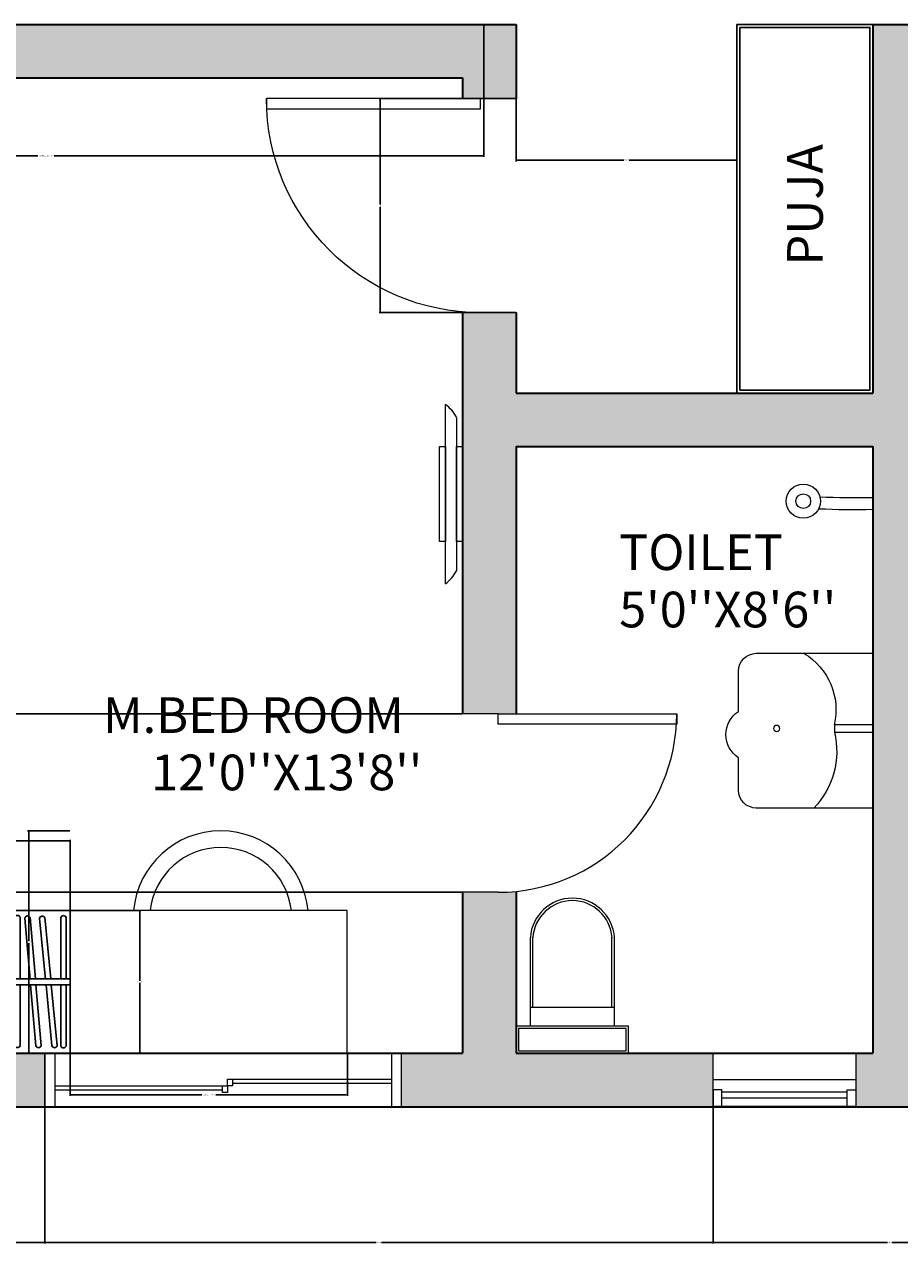
# Model space of a CAD drawing. Units: inches. Extents: x 1789 to 2841, y 3180 to 3702.
# Tile 9 of 14: x 2477 to 2624, y 3180 to 3385. Entities that reach past the tile are written whole.
import ezdxf

# ---------------------------------------------------------------- set-up
doc = ezdxf.new("R2010")
doc.units = ezdxf.units.IN
doc.header["$MEASUREMENT"] = 0
for name, color, linetype, lineweight in [('A-ANNO-DIMS', 2, 'Continuous', 18), ('A-AREA-IDEN', 7, 'Continuous', 18), ('A-EQPM', 8, 'Continuous', 18), ('A-FLOR-CASE', 34, 'Continuous', 25), ('A-FLOR-FIXT', 9, 'Continuous', 18), ('A-WALL', 40, 'Continuous', 35), ('A-WALL-PATT', 252, 'Continuous', 13), ('DORS', 70, 'Continuous', 18), ('FURNITURE', 34, 'Continuous', 18), ('WINDOWS', 130, 'Continuous', 18)]:
    doc.layers.add(name, color=color, linetype=linetype, lineweight=lineweight)
doc.styles.get("Standard").update_dxf_attribs({"font": 'arial.ttf'})
doc.dimstyles.get("Standard").update_dxf_attribs({"dimtxt": 0.18, "dimasz": 0.18, "dimexe": 0.18, "dimexo": 0.0625, "dimgap": 0.09, "dimtad": 0, "dimtih": 1, "dimtoh": 1, "dimdec": 0, "dimzin": 0, "dimdsep": 46, "dimlunit": 3, "dimtxsty": 'Standard', "dimcen": 0.09, "dimadec": 0, "dimazin": 0, "dimtfac": 1, "dimtdec": 0, "dimtofl": 0, "dimtmove": 0, "dimatfit": 3, "dimfxl": 1, "dimtolj": 1, "dimtzin": 0, "dimarcsym": 0})

# ---------------------------------------------------------------- blocks, each defined once
blk = doc.blocks.new('CUBOARD')
for p, q in [((2183.73, 3646.16), (2183.73, 3568.16)), ((2184.71, 3646.16), (2184.71, 3568.16))]:
    blk.add_line(p, q)
blk.add_lwpolyline([(2172.23, 3646.16), (2196.23, 3646.16), (2196.23, 3568.16), (2172.23, 3568.16)], close=True)
for points in [[(2195.39, 3645.6), (2184.67, 3644.55)], [(2183.69, 3644.46), (2173.95, 3643.51)], [(2173.97, 3642.61), (2183.78, 3643.57)], [(2184.76, 3643.66), (2195.54, 3644.71)], [(2195.78, 3645.16), (2195.78, 3645.18)], [(2183.73, 3641.98), (2173.93, 3641.98)], [(2195.47, 3641.98), (2184.71, 3641.98)], [(2195.82, 3641.5), (2195.82, 3641.53)], [(2173.86, 3641.08), (2183.73, 3641.08)], [(2183.76, 3639.46), (2173.96, 3640.08)], [(2184.71, 3641.08), (2195.53, 3641.08)], [(2195.45, 3638.71), (2184.74, 3639.4)], [(2173.84, 3639.19), (2183.7, 3638.57)], [(2184.68, 3638.5), (2195.46, 3637.81)], [(2195.77, 3638.22), (2195.78, 3638.24)], [(2173.83, 3635.92), (2183.73, 3635.92)], [(2183.73, 3636.82), (2173.9, 3636.82)], [(2195.43, 3636.82), (2184.71, 3636.82)], [(2184.71, 3635.92), (2195.5, 3635.92)], [(2195.78, 3636.35), (2195.78, 3636.37)], [(2173.81, 3633.34), (2183.73, 3633.34)], [(2183.73, 3634.24), (2173.88, 3634.24)], [(2195.42, 3634.24), (2184.71, 3634.24)], [(2184.71, 3633.34), (2195.48, 3633.34)], [(2195.77, 3633.77), (2195.77, 3633.79)], [(2183.73, 3631.66), (2173.86, 3631.66)], [(2195.4, 3631.66), (2184.71, 3631.66)], [(2195.75, 3631.19), (2195.75, 3631.21)], [(2173.8, 3630.76), (2183.73, 3630.76)], [(2184.71, 3630.76), (2195.47, 3630.76)], [(2173.78, 3628.19), (2183.73, 3628.19)], [(2183.73, 3629.08), (2173.85, 3629.08)], [(2183.8, 3626.57), (2173.93, 3627.31)], [(2195.38, 3629.08), (2184.71, 3629.08)], [(2184.71, 3628.19), (2195.45, 3628.19)], [(2195.73, 3628.61), (2195.73, 3628.63)], [(2173.79, 3626.43), (2183.74, 3625.68)], [(2184.71, 3625.61), (2195.4, 3624.81)], [(2195.4, 3625.7), (2184.78, 3626.5)], [(2195.72, 3625.21), (2195.72, 3625.23)], [(2173.75, 3623.03), (2183.73, 3623.03)], [(2183.73, 3623.92), (2173.81, 3623.92)], [(2195.35, 3623.92), (2184.71, 3623.92)], [(2184.71, 3623.03), (2195.42, 3623.03)], [(2195.7, 3623.45), (2195.7, 3623.48)], [(2183.73, 3621.34), (2173.8, 3621.34)], [(2195.33, 3621.34), (2184.71, 3621.34)], [(2173.73, 3620.45), (2183.73, 3620.45)], [(2195.22, 3619.57), (2184.65, 3618.76)], [(2184.71, 3620.45), (2195.4, 3620.45)], [(2195.6, 3619.13), (2195.6, 3619.15)], [(2195.68, 3620.87), (2195.68, 3620.9)], [(2183.67, 3618.69), (2173.75, 3617.93)], [(2173.75, 3617.03), (2183.74, 3617.8)], [(2184.71, 3617.87), (2195.35, 3618.68)], [(2173.7, 3615.29), (2183.73, 3615.29)], [(2183.73, 3616.19), (2173.77, 3616.19)], [(2195.3, 3616.19), (2184.71, 3616.19)], [(2184.71, 3615.29), (2195.37, 3615.29)], [(2195.65, 3615.71), (2195.65, 3615.74)], [(2173.68, 3612.71), (2183.73, 3612.71)], [(2183.73, 3613.61), (2173.75, 3613.61)], [(2195.28, 3613.61), (2184.71, 3613.61)], [(2184.71, 3612.71), (2195.35, 3612.71)], [(2195.63, 3613.14), (2195.63, 3613.16)], [(2173.67, 3611.18), (2183.69, 3610.23)], [(2183.78, 3611.12), (2173.82, 3612.07)], [(2195.26, 3610.03), (2184.75, 3611.03)], [(2184.67, 3610.14), (2195.24, 3609.13)], [(2195.23, 3608.76), (2184.7, 3608.45)], [(2195.56, 3609.53), (2195.57, 3609.55)], [(2173.66, 3607.23), (2183.75, 3607.53)], [(2183.72, 3608.42), (2173.71, 3608.13)], [(2184.73, 3607.55), (2195.33, 3607.87)], [(2195.6, 3608.3), (2195.6, 3608.32)], [(2173.63, 3604.98), (2183.73, 3604.98)], [(2183.73, 3605.87), (2173.7, 3605.87)], [(2195.23, 3605.87), (2184.71, 3605.87)], [(2184.71, 3604.98), (2195.3, 3604.98)], [(2195.58, 3605.4), (2195.58, 3605.42)], [(2183.73, 3603.29), (2173.68, 3603.29)], [(2195.22, 3603.29), (2184.71, 3603.29)], [(2195.57, 3602.82), (2195.57, 3602.84)], [(2173.61, 3602.4), (2183.73, 3602.4)], [(2183.73, 3600.71), (2173.67, 3600.71)], [(2184.71, 3602.4), (2195.28, 3602.4)], [(2195.2, 3600.71), (2184.71, 3600.71)], [(2173.6, 3599.82), (2183.73, 3599.82)], [(2184.71, 3599.82), (2195.27, 3599.82)], [(2195.55, 3600.24), (2195.55, 3600.27)], [(2173.58, 3597.24), (2183.73, 3597.24)], [(2183.73, 3598.13), (2173.65, 3598.13)], [(2195.18, 3598.13), (2184.71, 3598.13)], [(2184.71, 3597.24), (2195.25, 3597.24)], [(2195.53, 3597.66), (2195.53, 3597.69)], [(2173.56, 3595.36), (2183.71, 3594.72)], [(2183.77, 3595.62), (2173.68, 3596.25)], [(2184.69, 3594.66), (2195.19, 3594)], [(2195.18, 3594.9), (2184.74, 3595.55)], [(2195.5, 3594.4), (2195.5, 3594.43)], [(2183.73, 3592.98), (2173.62, 3592.98)], [(2195.15, 3592.98), (2184.71, 3592.98)], [(2195.5, 3592.5), (2195.5, 3592.53)], [(2173.55, 3592.08), (2183.73, 3592.08)], [(2173.57, 3590.49), (2183.74, 3589.59)], [(2183.73, 3590.49), (2173.72, 3591.37)], [(2184.71, 3592.08), (2195.22, 3592.08)], [(2195.17, 3589.47), (2184.71, 3590.4)], [(2184.71, 3589.5), (2195.16, 3588.58)], [(2195.48, 3588.97), (2195.48, 3589)], [(2173.51, 3586.92), (2183.73, 3586.92)], [(2183.73, 3587.82), (2173.58, 3587.82)], [(2194.84, 3586.83), (2184.58, 3585.23)], [(2195.12, 3587.82), (2184.71, 3587.82)], [(2184.71, 3586.92), (2195.19, 3586.92)], [(2195.26, 3586.41), (2195.25, 3586.44)], [(2195.47, 3587.35), (2195.47, 3587.37)], [(2183.61, 3585.08), (2173.56, 3583.51)], [(2173.63, 3582.62), (2183.75, 3584.19)], [(2184.71, 3584.34), (2195.04, 3585.95)], [(2183.73, 3582.66), (2173.55, 3582.66)], [(2195.08, 3582.66), (2184.71, 3582.66)], [(2195.43, 3582.19), (2195.43, 3582.21)], [(2173.48, 3581.77), (2183.73, 3581.77)], [(2183.73, 3580.08), (2173.53, 3580.08)], [(2184.71, 3581.77), (2195.15, 3581.77)], [(2195.07, 3580.08), (2184.71, 3580.08)], [(2173.46, 3579.19), (2183.73, 3579.19)], [(2184.71, 3579.19), (2195.14, 3579.19)], [(2195.42, 3579.61), (2195.42, 3579.63)], [(2173.45, 3576.61), (2183.73, 3576.61)], [(2183.73, 3577.5), (2173.52, 3577.5)], [(2194.92, 3575.81), (2184.64, 3574.92)], [(2195.05, 3577.5), (2184.71, 3577.5)], [(2184.71, 3576.61), (2195.12, 3576.61)], [(2195.4, 3577.03), (2195.4, 3577.05)], [(2183.66, 3574.84), (2173.46, 3573.95)], [(2173.47, 3573.05), (2183.74, 3573.94)], [(2184.71, 3574.03), (2195.06, 3574.93)], [(2195.31, 3575.37), (2195.31, 3575.4)], [(2183.65, 3572.24), (2173.45, 3571.25)], [(2194.88, 3573.34), (2184.63, 3572.34)], [(2184.71, 3571.45), (2195.04, 3572.46)], [(2195.28, 3572.91), (2195.27, 3572.93)], [(2173.47, 3570.35), (2183.74, 3571.35)], [(2183.73, 3569.77), (2173.47, 3569.77)], [(2195, 3569.77), (2184.71, 3569.77)], [(2173.4, 3568.87), (2183.73, 3568.87)], [(2184.71, 3568.87), (2195.07, 3568.87)], [(2195.35, 3569.29), (2195.35, 3569.32)]]:
    blk.add_lwpolyline(points)
for centre, start, end in [((2195.31, 3645.13), 7.0195, 80.386), ((2174.12, 3643.06), 110.7367, 251.6587), ((2195.31, 3645.13), 299.464, 4.1032), ((2174.06, 3641.52), 105.1753, 246.0974), ((2195.34, 3641.52), 1.4582, 74.8247), ((2195.34, 3641.52), 293.9026, 358.5418), ((2174.06, 3639.62), 101.5232, 242.4452), ((2195.3, 3638.26), 357.8061, 71.1726), ((2195.3, 3638.26), 290.2505, 354.8897), ((2174.02, 3636.36), 105.1753, 246.0974), ((2195.31, 3636.36), 1.4582, 74.8247), ((2195.31, 3636.36), 293.9026, 358.5418), ((2174.01, 3633.78), 105.1753, 246.0974), ((2195.29, 3633.78), 1.4582, 74.8247), ((2195.29, 3633.78), 293.9026, 358.5418), ((2173.99, 3631.2), 105.1753, 246.0974), ((2195.27, 3631.2), 1.4582, 74.8247), ((2195.27, 3631.2), 293.9026, 358.5418), ((2173.97, 3628.62), 105.1753, 246.0974), ((2174.02, 3626.85), 100.888, 241.81), ((2195.26, 3628.62), 1.4582, 74.8247), ((2195.26, 3628.62), 293.9026, 358.5418), ((2195.24, 3625.25), 357.1709, 70.5374), ((2195.24, 3625.25), 289.6153, 354.2545), ((2173.94, 3623.46), 105.1753, 246.0974), ((2195.22, 3623.46), 1.4582, 74.8247), ((2195.22, 3623.46), 293.9026, 358.5418), ((2173.92, 3620.88), 105.1753, 246.0974), ((2195.21, 3620.88), 1.4582, 74.8247), ((2195.13, 3619.1), 5.8369, 79.2034), ((2195.13, 3619.1), 298.2814, 2.9206), ((2195.21, 3620.88), 293.9026, 358.5418), ((2173.9, 3617.48), 109.5541, 250.4761), ((2173.89, 3615.73), 105.1753, 246.0974), ((2195.17, 3615.73), 1.4582, 74.8247), ((2195.17, 3615.73), 293.9026, 358.5418), ((2173.87, 3613.15), 105.1753, 246.0974), ((2195.16, 3613.15), 1.4582, 74.8247), ((2195.16, 3613.15), 293.9026, 358.5418), ((2173.9, 3611.6), 99.7479, 240.6699), ((2195.12, 3608.3), 3.1408, 76.5073), ((2195.09, 3609.58), 288.4752, 353.1144), ((2195.09, 3609.58), 356.0307, 69.3973), ((2173.84, 3607.67), 106.858, 247.78), ((2195.12, 3608.3), 295.5853, 0.2245), ((2173.82, 3605.41), 105.1753, 246.0974), ((2195.11, 3605.41), 1.4582, 74.8247), ((2195.11, 3605.41), 293.9026, 358.5418), ((2173.81, 3602.83), 105.1753, 246.0974), ((2195.09, 3602.83), 1.4582, 74.8247), ((2195.09, 3602.83), 293.9026, 358.5418), ((2173.79, 3600.25), 105.1753, 246.0974), ((2195.08, 3600.25), 1.4582, 74.8247), ((2195.08, 3600.25), 293.9026, 358.5418), ((2173.77, 3597.67), 105.1753, 246.0974), ((2195.06, 3597.67), 1.4582, 74.8247), ((2195.06, 3597.67), 293.9026, 358.5418), ((2173.78, 3595.78), 101.566, 242.4881), ((2195.02, 3594.44), 357.8489, 71.2154), ((2195.02, 3594.44), 290.2933, 354.9325), ((2173.74, 3592.52), 105.1753, 246.0974), ((2195.03, 3592.52), 1.4582, 74.8247), ((2195.03, 3592.52), 293.9026, 358.5418), ((2173.8, 3590.9), 100.1162, 241.0382), ((2195.01, 3589.03), 288.8435, 353.4827), ((2195.01, 3589.03), 356.399, 69.7655), ((2173.71, 3587.36), 105.1753, 246.0974), ((2194.79, 3586.35), 10.3063, 83.6728), ((2194.79, 3586.35), 302.7507, 7.3899), ((2194.99, 3587.36), 1.4582, 74.8247), ((2194.99, 3587.36), 293.9026, 358.5418), ((2173.67, 3582.2), 105.1753, 246.0974), ((2173.75, 3583.08), 114.0234, 254.9455), ((2194.96, 3582.2), 1.4582, 74.8247), ((2194.96, 3582.2), 293.9026, 358.5418), ((2173.66, 3579.62), 105.1753, 246.0974), ((2194.94, 3579.62), 1.4582, 74.8247), ((2194.94, 3579.62), 293.9026, 358.5418), ((2173.64, 3577.04), 105.1753, 246.0974), ((2194.83, 3575.34), 6.4142, 79.7807), ((2194.93, 3577.04), 1.4582, 74.8247), ((2194.93, 3577.04), 293.9026, 358.5418), ((2173.63, 3573.5), 110.1314, 251.0534), ((2194.83, 3575.34), 298.8587, 3.4979), ((2194.8, 3572.87), 7.0476, 80.4142), ((2194.8, 3572.87), 299.4921, 4.1313), ((2173.59, 3569.31), 105.1753, 246.0974), ((2173.62, 3570.8), 110.7648, 251.6868), ((2194.88, 3569.31), 1.4582, 74.8247), ((2194.88, 3569.31), 293.9026, 358.5418)]:
    blk.add_arc(centre, 0.476, start, end)
blk = doc.blocks.new('KIKI')
blk.add_lwpolyline([(2076.233, 3621.086), (2067.627, 3621.086), (2067.627, 3604.375), (2076.233, 3604.375)], close=True)
for radius, start, end in [(5.285, 95.30288, 264.69712), (4.285, 96.54542, 263.45458)]:
    blk.add_arc((2068.115, 3613.452), radius, start, end)
blk = doc.blocks.new('HYJ')
for p, q in [((2206.12, 3649.67), (2234.3, 3649.67)), ((2236.02, 3650.77), (2262.74, 3650.77)), ((2236.02, 3650.11), (2262.74, 3650.11)), ((2206.12, 3649), (2234.3, 3649))]:
    blk.add_line(p, q)
for points in [[(2204.43, 3646.16), (2264.43, 3646.16), (2264.43, 3655.16), (2204.43, 3655.16)], [(2204.43, 3655.16), (2206.12, 3655.16), (2206.12, 3646.16), (2204.43, 3646.16)], [(2264.43, 3655.16), (2262.74, 3655.16), (2262.74, 3646.16), (2264.43, 3646.16)], [(2234.3, 3649.67), (2235.16, 3649.67), (2235.16, 3648.56), (2234.3, 3648.56)], [(2235.16, 3650.77), (2236.02, 3650.77), (2236.02, 3649.67), (2235.16, 3649.67)]]:
    blk.add_lwpolyline(points, close=True)
blk = doc.blocks.new('*U9')
for p, q in [((0, 0), (0, -6)), ((36, 0), (36, -6))]:
    blk.add_line(p, q)
blk.add_lwpolyline([(0, 0), (0, 36), (1.75, 36), (1.75, 0)], close=True)
blk.add_arc((0, 0), 36, 0, 90)
blk = doc.blocks.new('GTGTG')
for points in [[(2266.82, 3646.16), (2282.82, 3646.16), (2282.82, 3645.14), (2266.82, 3645.14)], [(2266.82, 3643.29), (2282.82, 3643.29), (2282.82, 3642.27), (2266.82, 3642.27)]]:
    blk.add_lwpolyline(points, close=True)
for points in [[(2261.92, 3645.14), (2287.72, 3645.14)], [(2289.9, 3643.29), (2259.74, 3643.29)]]:
    blk.add_lwpolyline(points)
for centre, start, end in [((2265.21, 3639.05), 118.4184, 142.2436), ((2284.43, 3639.05), 37.7564, 61.5816)]:
    blk.add_arc(centre, 6.92, start, end)
blk = doc.blocks.new('*U10')
for p, q in [((0, 0), (0, -6)), ((30, 0), (30, -6))]:
    blk.add_line(p, q)
blk.add_lwpolyline([(0, 0), (0, 30), (1.75, 30), (1.75, 0)], close=True)
blk.add_arc((0, 0), 30, 0, 90)
blk = doc.blocks.new('HY')
for p, q in [((2053.67, 3653.75), (2074.8, 3653.75)), ((2053.67, 3652.75), (2074.8, 3652.75)), ((2052.23, 3650.66), (2076.23, 3650.66))]:
    blk.add_line(p, q)
for points in [[(2076.23, 3646.16), (2052.23, 3646.16), (2052.23, 3655.16), (2076.23, 3655.16)], [(2052.23, 3655.16), (2053.67, 3655.16), (2053.67, 3652.35), (2052.23, 3652.35)], [(2076.23, 3655.16), (2074.8, 3655.16), (2074.8, 3652.35), (2076.23, 3652.35)]]:
    blk.add_lwpolyline(points, close=True)
blk = doc.blocks.new('GT')
for p, q in [((2141.38, 3640.15), (2141.38, 3620.49)), ((2160.08, 3640.15), (2160.08, 3620.49)), ((2141.38, 3636.04), (2160.08, 3636.04)), ((2141.93, 3636.04), (2141.93, 3620.49)), ((2159.53, 3636.04), (2159.53, 3620.49))]:
    blk.add_line(p, q)
for points in [[(2163.23, 3646.16), (2138.23, 3646.16), (2138.23, 3640.15), (2163.23, 3640.15)], [(2162.68, 3645.61), (2138.78, 3645.61), (2138.78, 3640.7), (2162.68, 3640.7)]]:
    blk.add_lwpolyline(points, close=True)
for radius in [9.37, 8.82]:
    blk.add_arc((2150.73, 3621.09), radius, 183.6546, 356.3454)
blk = doc.blocks.new('TYTY')
for p, q in [((2104.84, 3607.68), (2085.23, 3607.68)), ((2085.23, 3607.68), (2085.23, 3581.66)), ((2107.84, 3597.9), (2107.84, 3604.68)), ((2107.84, 3584.66), (2107.84, 3590.13)), ((2085.23, 3581.66), (2104.84, 3581.66))]:
    blk.add_line(p, q)
blk.add_lwpolyline([(2085.23, 3595.66), (2091.71, 3595.66), (2091.71, 3594.41), (2085.23, 3594.41)], close=True)
blk.add_circle((2101.42, 3595.04), 0.517)
for centre, radius, start, end in [((2102.58, 3598.14), 11.14, 121.1396, 192.8397), ((2104.84, 3604.68), 3, 0, 90), ((2105.34, 3594.01), 4.62, 302.7804, 57.2196), ((2104.89, 3591.14), 13.58, 166.0641, 224.2681), ((2104.84, 3584.66), 3, 270, 0)]:
    blk.add_arc(centre, radius, start, end)
blk = doc.blocks.new('SOUW')
for radius in [2.88, 1.24]:
    blk.add_circle((2096.93, 3622.15), radius)
for radius, start in [(130.14, 87.3378), (128.14, 87.3891)]:
    blk.add_arc((2088.3, 3493.42), radius, start, 91.3578)
blk = doc.blocks.new('*D37')
at = {"layer": 'A-ANNO-DIMS', "color": 0, "lineweight": -2, "transparency": 16777216}
for p, q in [((2406.23, 3236.22), (2406.23, 3248.04)), ((2406.41, 3247.86), (2443.93, 3247.86)), ((2484.05, 3247.86), (2446.54, 3247.86)), ((2484.23, 3236.22), (2484.23, 3248.04))]:
    blk.add_line(p, q, dxfattribs=at)
at = {"layer": 'A-ANNO-DIMS', "color": 0, "transparency": 16777216}
for points in [[(2406.41, 3247.89), (2406.41, 3247.83), (2406.23, 3247.86)], [(2484.05, 3247.89), (2484.05, 3247.83), (2484.23, 3247.86)]]:
    blk.add_solid(points, dxfattribs=at)
at = {"layer": 'Defpoints', "color": 0, "transparency": 16777216}
for p in [(2406.23, 3247.86), (2406.23, 3236.16), (2484.23, 3236.16)]:
    blk.add_point(p, dxfattribs=at)
at = {"layer": 'A-ANNO-DIMS', "color": 0, "transparency": 16777216, "insert": (2445.23, 3247.86), "char_height": 0.18, "attachment_point": 5}
blk.add_mtext('\\A1;WARDROBE 78 TYP.', dxfattribs=at)
blk = doc.blocks.new('*D38')
at = {"layer": 'A-ANNO-DIMS', "color": 0, "lineweight": -2, "transparency": 16777216}
for p, q in [((2484.3, 3236.16), (2496.11, 3236.16)), ((2495.93, 3235.98), (2495.93, 3224.34)), ((2495.93, 3212.34), (2495.93, 3223.98)), ((2484.3, 3212.16), (2496.11, 3212.16))]:
    blk.add_line(p, q, dxfattribs=at)
at = {"layer": 'A-ANNO-DIMS', "color": 0, "transparency": 16777216}
for points in [[(2495.9, 3235.98), (2495.96, 3235.98), (2495.93, 3236.16)], [(2495.9, 3212.34), (2495.96, 3212.34), (2495.93, 3212.16)]]:
    blk.add_solid(points, dxfattribs=at)
at = {"layer": 'Defpoints', "color": 0, "transparency": 16777216}
for p in [(2484.23, 3236.16), (2495.93, 3236.16), (2484.23, 3212.16)]:
    blk.add_point(p, dxfattribs=at)
at = {"layer": 'A-ANNO-DIMS', "color": 0, "transparency": 16777216, "insert": (2495.93, 3224.16), "char_height": 0.18, "attachment_point": 5}
blk.add_mtext('\\A1;24 TYP.', dxfattribs=at)
blk = doc.blocks.new('*D49')
at = {"layer": 'A-ANNO-DIMS', "color": 0, "lineweight": -2, "transparency": 16777216}
for p, q in [((2484.23, 3212.1), (2484.23, 3204.99)), ((2530.84, 3212.1), (2530.84, 3204.99)), ((2484.41, 3205.17), (2506.35, 3205.17)), ((2530.66, 3205.17), (2508.72, 3205.17))]:
    blk.add_line(p, q, dxfattribs=at)
at = {"layer": 'A-ANNO-DIMS', "color": 0, "transparency": 16777216}
for points in [[(2484.41, 3205.2), (2484.41, 3205.14), (2484.23, 3205.17)], [(2530.66, 3205.2), (2530.66, 3205.14), (2530.84, 3205.17)]]:
    blk.add_solid(points, dxfattribs=at)
at = {"layer": 'Defpoints', "color": 0, "transparency": 16777216}
for p in [(2484.23, 3212.16), (2530.84, 3212.16), (2530.84, 3205.17)]:
    blk.add_point(p, dxfattribs=at)
at = {"layer": 'A-ANNO-DIMS', "color": 0, "transparency": 16777216, "insert": (2507.53, 3205.17), "char_height": 0.18, "attachment_point": 5}
blk.add_mtext('\\A1;DESK SET 47 TYP.', dxfattribs=at)
blk = doc.blocks.new('*D50')
at = {"layer": 'A-ANNO-DIMS', "color": 0, "lineweight": -2, "transparency": 16777216}
for p, q in [((2484.17, 3249.54), (2477.06, 3249.54)), ((2477.24, 3249.36), (2477.24, 3231.03)), ((2477.24, 3212.34), (2477.24, 3230.67)), ((2484.17, 3212.16), (2477.06, 3212.16))]:
    blk.add_line(p, q, dxfattribs=at)
at = {"layer": 'A-ANNO-DIMS', "color": 0, "transparency": 16777216}
for points in [[(2477.21, 3249.36), (2477.27, 3249.36), (2477.24, 3249.54)], [(2477.21, 3212.34), (2477.27, 3212.34), (2477.24, 3212.16)]]:
    blk.add_solid(points, dxfattribs=at)
at = {"layer": 'Defpoints', "color": 0, "transparency": 16777216}
for p in [(2484.23, 3249.54), (2477.24, 3212.16), (2484.23, 3212.16)]:
    blk.add_point(p, dxfattribs=at)
at = {"layer": 'A-ANNO-DIMS', "color": 0, "transparency": 16777216, "insert": (2477.24, 3230.85), "char_height": 0.18, "attachment_point": 5}
blk.add_mtext('\\A1;37 TYP.', dxfattribs=at)
blk = doc.blocks.new('*D69')
at = {"layer": 'A-ANNO-DIMS', "color": 0, "lineweight": -2, "transparency": 16777216}
for p, q in [((2406.54, 3385.11), (2406.54, 3362.9)), ((2553.79, 3385.11), (2553.79, 3362.9)), ((2406.72, 3363.08), (2478.8, 3363.08)), ((2553.61, 3363.08), (2481.54, 3363.08))]:
    blk.add_line(p, q, dxfattribs=at)
at = {"layer": 'A-ANNO-DIMS', "color": 0, "transparency": 16777216}
for points in [[(2406.72, 3363.11), (2406.72, 3363.05), (2406.54, 3363.08)], [(2553.61, 3363.11), (2553.61, 3363.05), (2553.79, 3363.08)]]:
    blk.add_solid(points, dxfattribs=at)
at = {"layer": 'Defpoints', "color": 0, "transparency": 16777216}
for p in [(2406.54, 3385.17), (2553.79, 3385.17), (2553.79, 3363.08)]:
    blk.add_point(p, dxfattribs=at)
at = {"layer": 'A-ANNO-DIMS', "color": 0, "transparency": 16777216, "insert": (2480.17, 3363.08), "char_height": 0.18, "attachment_point": 5}
blk.add_mtext('\\A1;SEATING GROUP 147', dxfattribs=at)
blk = doc.blocks.new('*D97')
at = {"layer": 'A-ANNO-DIMS', "color": 0, "lineweight": -2, "transparency": 16777216}
for p, q in [((2397.23, 3203.1), (2397.23, 3180.13)), ((2479.95, 3203.1), (2479.95, 3180.13)), ((2397.41, 3180.31), (2438.2, 3180.31)), ((2479.77, 3180.31), (2438.98, 3180.31))]:
    blk.add_line(p, q, dxfattribs=at)
at = {"layer": 'A-ANNO-DIMS', "color": 0, "transparency": 16777216}
for points in [[(2397.41, 3180.34), (2397.41, 3180.28), (2397.23, 3180.31)], [(2479.77, 3180.34), (2479.77, 3180.28), (2479.95, 3180.31)]]:
    blk.add_solid(points, dxfattribs=at)
at = {"layer": 'Defpoints', "color": 0, "transparency": 16777216}
for p in [(2397.23, 3203.16), (2479.95, 3203.16), (2479.95, 3180.31)]:
    blk.add_point(p, dxfattribs=at)
at = {"layer": 'A-ANNO-DIMS', "color": 0, "transparency": 16777216, "insert": (2438.59, 3180.31), "char_height": 0.18, "attachment_point": 5}
blk.add_mtext('\\A1;82.72', dxfattribs=at)
blk = doc.blocks.new('*D98')
at = {"layer": 'A-ANNO-DIMS', "color": 0, "lineweight": -2, "transparency": 16777216}
for p, q in [((2479.95, 3203.1), (2479.95, 3180.13)), ((2592.37, 3203.1), (2592.37, 3180.13)), ((2480.13, 3180.31), (2535.71, 3180.31)), ((2592.19, 3180.31), (2536.61, 3180.31))]:
    blk.add_line(p, q, dxfattribs=at)
at = {"layer": 'A-ANNO-DIMS', "color": 0, "transparency": 16777216}
for points in [[(2480.13, 3180.34), (2480.13, 3180.28), (2479.95, 3180.31)], [(2592.19, 3180.34), (2592.19, 3180.28), (2592.37, 3180.31)]]:
    blk.add_solid(points, dxfattribs=at)
at = {"layer": 'Defpoints', "color": 0, "transparency": 16777216}
for p in [(2479.95, 3203.16), (2592.37, 3203.16), (2592.37, 3180.31)]:
    blk.add_point(p, dxfattribs=at)
at = {"layer": 'A-ANNO-DIMS', "color": 0, "transparency": 16777216, "insert": (2536.16, 3180.31), "char_height": 0.18, "attachment_point": 5}
blk.add_mtext('\\A1;112.42', dxfattribs=at)
blk = doc.blocks.new('*D99')
at = {"layer": 'A-ANNO-DIMS', "color": 0, "lineweight": -2, "transparency": 16777216}
for p, q in [((2592.37, 3203.1), (2592.37, 3180.13)), ((2651.85, 3203.1), (2651.85, 3180.13)), ((2592.55, 3180.31), (2621.72, 3180.31)), ((2651.67, 3180.31), (2622.5, 3180.31))]:
    blk.add_line(p, q, dxfattribs=at)
at = {"layer": 'A-ANNO-DIMS', "color": 0, "transparency": 16777216}
for points in [[(2592.55, 3180.34), (2592.55, 3180.28), (2592.37, 3180.31)], [(2651.67, 3180.34), (2651.67, 3180.28), (2651.85, 3180.31)]]:
    blk.add_solid(points, dxfattribs=at)
at = {"layer": 'Defpoints', "color": 0, "transparency": 16777216}
for p in [(2592.37, 3203.16), (2651.85, 3203.16), (2651.85, 3180.31)]:
    blk.add_point(p, dxfattribs=at)
at = {"layer": 'A-ANNO-DIMS', "color": 0, "transparency": 16777216, "insert": (2622.11, 3180.31), "char_height": 0.18, "attachment_point": 5}
blk.add_mtext('\\A1;59.48', dxfattribs=at)
blk = doc.blocks.new('*D109')
at = {"layer": 'A-ANNO-DIMS', "color": 0, "lineweight": -2, "transparency": 16777216}
for p, q in [((2559.17, 3372.69), (2536.2, 3372.69)), ((2536.38, 3372.51), (2536.38, 3354.87)), ((2536.38, 3336.87), (2536.38, 3354.51)), ((2559.17, 3336.69), (2536.2, 3336.69))]:
    blk.add_line(p, q, dxfattribs=at)
at = {"layer": 'A-ANNO-DIMS', "color": 0, "transparency": 16777216}
for points in [[(2536.35, 3372.51), (2536.41, 3372.51), (2536.38, 3372.69)], [(2536.35, 3336.87), (2536.41, 3336.87), (2536.38, 3336.69)]]:
    blk.add_solid(points, dxfattribs=at)
at = {"layer": 'Defpoints', "color": 0, "transparency": 16777216}
for p in [(2536.38, 3372.69), (2559.23, 3372.69), (2559.23, 3336.69)]:
    blk.add_point(p, dxfattribs=at)
at = {"layer": 'A-ANNO-DIMS', "color": 0, "transparency": 16777216, "insert": (2536.38, 3354.69), "char_height": 0.18, "attachment_point": 5}
blk.add_mtext('\\A1;36', dxfattribs=at)
blk = doc.blocks.new('*D110')
at = {"layer": 'A-ANNO-DIMS', "color": 0, "lineweight": -2, "transparency": 16777216}
for p, q in [((2550.17, 3269.21), (2374.2, 3269.21)), ((2374.38, 3269.03), (2374.38, 3254.4)), ((2374.38, 3239.39), (2374.38, 3254.03)), ((2550.17, 3239.21), (2374.2, 3239.21))]:
    blk.add_line(p, q, dxfattribs=at)
at = {"layer": 'A-ANNO-DIMS', "color": 0, "transparency": 16777216}
for points in [[(2374.35, 3269.03), (2374.41, 3269.03), (2374.38, 3269.21)], [(2374.35, 3239.39), (2374.41, 3239.39), (2374.38, 3239.21)]]:
    blk.add_solid(points, dxfattribs=at)
at = {"layer": 'Defpoints', "color": 0, "transparency": 16777216}
for p in [(2374.38, 3269.21), (2550.23, 3269.21), (2550.23, 3239.21)]:
    blk.add_point(p, dxfattribs=at)
at = {"layer": 'A-ANNO-DIMS', "color": 0, "transparency": 16777216, "insert": (2374.38, 3254.21), "char_height": 0.18, "attachment_point": 5}
blk.add_mtext('\\A1;30', dxfattribs=at)
blk = doc.blocks.new('*D111')
at = {"layer": 'A-ANNO-DIMS', "color": 0, "lineweight": -2, "transparency": 16777216}
for p, q in [((2559.23, 3385.1), (2559.23, 3362.13)), ((2596.36, 3385.1), (2596.36, 3362.13)), ((2559.41, 3362.31), (2577.33, 3362.31)), ((2596.18, 3362.31), (2578.26, 3362.31))]:
    blk.add_line(p, q, dxfattribs=at)
at = {"layer": 'A-ANNO-DIMS', "color": 0, "transparency": 16777216}
for points in [[(2559.41, 3362.34), (2559.41, 3362.28), (2559.23, 3362.31)], [(2596.18, 3362.34), (2596.18, 3362.28), (2596.36, 3362.31)]]:
    blk.add_solid(points, dxfattribs=at)
at = {"layer": 'Defpoints', "color": 0, "transparency": 16777216}
for p in [(2559.23, 3385.16), (2596.36, 3385.16), (2559.23, 3362.31)]:
    blk.add_point(p, dxfattribs=at)
at = {"layer": 'A-ANNO-DIMS', "color": 0, "transparency": 16777216, "insert": (2577.8, 3362.31), "char_height": 0.18, "attachment_point": 5}
blk.add_mtext('\\A1;37.125', dxfattribs=at)

msp = doc.modelspace()

# ---------------------------------------------------------------- hatches: boundary and pattern name
at = {"layer": 'A-WALL-PATT'}
h = msp.add_hatch(color=256, dxfattribs=at)
h.dxf.hatch_style = 1
edge = h.paths.add_edge_path()
edge.add_line((2559.2333, 3385.1608), (2442.3717, 3385.1608))
edge.add_line((2442.3717, 3385.1608), (2442.3717, 3385.1524))
edge.add_line((2442.3717, 3385.1524), (2418.8108, 3385.1608))
edge.add_line((2418.8108, 3385.1608), (2406.2333, 3385.1608))
edge.add_line((2406.2333, 3385.1608), (2406.5667, 3473.2999))
edge.add_arc((2403.2333, 3513.1608), 40, 270, 274.780192, ccw=False)
edge.add_line((2403.2333, 3473.1608), (2397.2333, 3473.1608))
edge.add_line((2397.2333, 3473.1608), (2397.2333, 3376.1608))
edge.add_line((2397.2333, 3376.1608), (2550.2333, 3376.1608))
edge.add_line((2550.2333, 3376.1608), (2550.2333, 3372.6905))
edge.add_arc((2551.7333, 3408.5966), 35.9374, 267.607822, 272.392178)
edge.add_line((2553.2333, 3372.6905), (2559.2333, 3372.6905))
edge.add_line((2559.2333, 3372.6905), (2559.2333, 3385.1608))
h = msp.add_hatch(color=256, dxfattribs=at)
h.dxf.hatch_style = 1
h.paths.add_polyline_path([(2628.2333, 3376.1608), (2657.1973, 3376.1608), (2657.1973, 3385.1608), (2619.2333, 3385.1608), (2619.2333, 3212.1608), (2616.3707, 3212.1608), (2616.3707, 3203.1608), (2651.8514, 3203.1608), (2651.8514, 3212.1608), (2628.2333, 3212.1608)])
h = msp.add_hatch(color=256, dxfattribs=at)
h.dxf.hatch_style = 1
edge = h.paths.add_edge_path()
edge.add_line((2559.2333, 3323.1608), (2559.2333, 3336.6905))
edge.add_line((2559.2333, 3336.6905), (2553.2333, 3336.6905))
edge.add_arc((2553.2333, 3372.6905), 36, 265.212633, 270, ccw=False)
edge.add_line((2550.2288, 3336.8161), (2550.2333, 3269.2132))
edge.add_line((2550.2333, 3269.2132), (2556.2333, 3269.2132))
edge.add_line((2556.2333, 3269.2132), (2559.2333, 3269.2132))
edge.add_line((2559.2333, 3269.2132), (2559.2333, 3314.1608))
edge.add_line((2559.2333, 3314.1608), (2619.2333, 3314.1608))
edge.add_line((2619.2333, 3314.1608), (2619.2333, 3323.1608))
edge.add_line((2619.2333, 3323.1608), (2596.3581, 3323.1608))
edge.add_line((2596.3581, 3323.1608), (2559.2333, 3323.1608))
h = msp.add_hatch(color=256, dxfattribs=at)
h.dxf.hatch_style = 1
h.paths.add_polyline_path([(2592.3707, 3212.1608), (2559.2333, 3212.1608), (2559.2333, 3216.7108), (2559.2333, 3239.3636, -0.02504709), (2556.2333, 3239.2132), (2550.2333, 3239.2132), (2550.2333, 3212.1608), (2539.9504, 3212.1608), (2539.9504, 3203.1608), (2592.3707, 3203.1608)])
h.paths.add_polyline_path([(2479.9504, 3212.1608), (2406.2333, 3212.1608), (2406.2333, 3236.1608), (2397.2333, 3236.1608), (2397.2333, 3203.1608), (2479.9504, 3203.1608)])

# ---------------------------------------------------------------- linework, layer by layer
at = {"layer": 'A-FLOR-CASE'}
for points in [[(2596.3581, 3385.1608), (2619.2333, 3385.1608), (2619.2333, 3323.1608), (2596.3581, 3323.1608)], [(2596.8581, 3384.6608), (2618.7333, 3384.6608), (2618.7333, 3323.6608), (2596.8581, 3323.6608)]]:
    msp.add_lwpolyline(points, close=True, dxfattribs=at)
at = {"layer": 'A-WALL'}
for p, q in [((2406.2333, 3385.1608), (2559.2333, 3385.1608)), ((2559.2333, 3385.1608), (2559.2333, 3372.6905)), ((2619.2333, 3385.1608), (2619.2333, 3323.1608)), ((2619.2333, 3385.1608), (2619.2333, 3376.1608)), ((2619.2333, 3385.1608), (2657.1973, 3385.1608)), ((2406.2333, 3376.1608), (2550.2333, 3376.1608)), ((2550.2333, 3376.1608), (2550.2333, 3372.6905)), ((2550.2288, 3336.8161), (2550.2333, 3269.2132)), ((2559.2333, 3336.6905), (2559.2333, 3323.1608)), ((2559.2333, 3323.1608), (2619.2333, 3323.1608)), ((2559.2333, 3314.1608), (2559.2333, 3269.2132)), ((2559.2333, 3314.1608), (2619.2333, 3314.1608)), ((2619.2333, 3314.1608), (2619.2333, 3212.1608)), ((2550.2333, 3239.2132), (2550.2333, 3212.1608)), ((2559.2333, 3239.3636), (2559.2333, 3212.1608)), ((2406.2333, 3212.1608), (2550.2333, 3212.1608)), ((2559.2333, 3212.1608), (2619.2333, 3212.1608)), ((2397.2333, 3203.1608), (2763.2333, 3203.1608))]:
    msp.add_line(p, q, dxfattribs=at)

# ---------------------------------------------------------------- block references
at = {"layer": 'A-EQPM', "rotation": 270}
msp.add_blockref('GTGTG', (-1095.9274, 5581.0033), dxfattribs=at)
at = {"layer": 'A-FLOR-CASE', "rotation": 90}
msp.add_blockref('CUBOARD', (6052.3941, 1039.9274), dxfattribs=at)
at = {"layer": 'A-FLOR-FIXT', "rotation": 180}
msp.add_blockref('SOUW', (4704.4533, 6927.1407), dxfattribs=at)
at = {"layer": 'A-FLOR-FIXT', "xscale": -1}
msp.add_blockref('TYTY', (4704.4667, -328.2819), dxfattribs=at)
at = {"layer": 'A-FLOR-FIXT', "xscale": 0.756665822373692, "yscale": 0.756665822373692, "zscale": 0.756665822373692, "rotation": 179.9999999999993}
msp.add_blockref('GT', (4196.0781, 5971.086), dxfattribs=at)
at = {"layer": 'DORS', "xscale": -1, "rotation": 90}
msp.add_blockref('*U9', (2553.2333, 3372.6905), dxfattribs=at)
at = {"layer": 'DORS', "rotation": 270}
msp.add_blockref('*U10', (2556.2333, 3269.2132), dxfattribs=at)
at = {"layer": 'FURNITURE', "xscale": 2.788618734312648, "yscale": 2.788618734312648, "zscale": 2.788618734312648, "rotation": 270}
msp.add_blockref('KIKI', (-7566.9935, 9001.984), dxfattribs=at)
at = {"layer": 'WINDOWS'}
msp.add_blockref('HYJ', (275.5179, -443), dxfattribs=at)
at = {"layer": 'WINDOWS', "rotation": 180}
msp.add_blockref('HY', (4668.604, 6858.3216), dxfattribs=at)

# ---------------------------------------------------------------- texts
at = {"layer": 'A-ANNO-DIMS'}
for s, p in [("5'0''X8'6''", (2576.5619, 3283.7619)), ("12'0''X13'8''", (2497.8453, 3256.3681))]:
    msp.add_text(s, height=6, dxfattribs=at).set_placement(p)
at = {"layer": 'A-AREA-IDEN'}
msp.add_text('PUJA', height=6, rotation=90, dxfattribs=at).set_placement((2610.812, 3344.6141))
for s, p in [('TOILET', (2576.5619, 3293.4004)), ('M.BED ROOM', (2489.7614, 3266.0066))]:
    msp.add_text(s, height=6, dxfattribs=at).set_placement(p)

# ---------------------------------------------------------------- dimensions: what is measured, and where the dimension line sits
at = {"layer": 'A-ANNO-DIMS'}
for base, p1, p2, text, picture, middle in [((2553.7897, 3363.0817), (2406.5443, 3385.1685), (2553.7897, 3385.1685), 'SEATING GROUP <>', '*D69', (2480.167, 3363.0817)), ((2530.8361, 3205.1704), (2484.2333, 3212.1608), (2530.8361, 3212.1608), 'DESK SET <> TYP.', '*D49', (2507.5347, 3205.1704))]:
    dim = msp.add_linear_dim(base=base, p1=p1, p2=p2, text=text, dimstyle='Standard', override={"dimdec": 0, "dimlfac": 1, "dimrnd": 0, "dimzin": 0, "dimdsep": 46, "dimlunit": 2}, dxfattribs=at)
    dim.commit()
    dim.dimension.update_dxf_attribs({"geometry": picture, "text_midpoint": middle})
for base, p1, p2, angle, override, picture, middle in [((2559.2333, 3362.3108), (2596.3581, 3385.1608), (2559.2333, 3385.1608), 180, {"dimdec": 3, "dimlfac": 1, "dimrnd": 0, "dimzin": 0, "dimdsep": 46, "dimlunit": 2}, '*D111', (2577.7957, 3362.3108)), ((2536.3833, 3372.6905), (2559.2333, 3336.6905), (2559.2333, 3372.6905), 90, {"dimdec": 0, "dimlfac": 1, "dimrnd": 0, "dimzin": 0, "dimdsep": 46, "dimlunit": 2}, '*D109', (2536.3833, 3354.6905)), ((2374.3833, 3269.2132), (2550.2333, 3239.2132), (2550.2333, 3269.2132), 90, {"dimdec": 0, "dimlfac": 1, "dimrnd": 0, "dimzin": 0, "dimdsep": 46, "dimlunit": 2}, '*D110', (2374.3833, 3254.2132))]:
    dim = msp.add_linear_dim(base=base, p1=p1, p2=p2, angle=angle, dimstyle='Standard', override=override, dxfattribs=at)
    dim.commit()
    dim.dimension.update_dxf_attribs({"geometry": picture, "text_midpoint": middle})
for base, p1, p2, angle, text, picture, middle in [((2406.2333, 3247.8608), (2484.2333, 3236.1608), (2406.2333, 3236.1608), 180, 'WARDROBE <> TYP.', '*D37', (2445.2333, 3247.8608)), ((2477.2429, 3212.1608), (2484.2333, 3249.5356), (2484.2333, 3212.1608), 270, '<> TYP.', '*D50', (2477.2429, 3230.8482)), ((2495.9333, 3236.1608), (2484.2333, 3212.1608), (2484.2333, 3236.1608), 90, '<> TYP.', '*D38', (2495.9333, 3224.1608))]:
    dim = msp.add_linear_dim(base=base, p1=p1, p2=p2, angle=angle, text=text, dimstyle='Standard', override={"dimdec": 0, "dimlfac": 1, "dimrnd": 0, "dimzin": 0, "dimdsep": 46, "dimlunit": 2}, dxfattribs=at)
    dim.commit()
    dim.dimension.update_dxf_attribs({"geometry": picture, "text_midpoint": middle})
for base, p1, p2, picture, middle in [((2479.9504, 3180.3108), (2397.2333, 3203.1608), (2479.9504, 3203.1608), '*D97', (2438.5919, 3180.3108)), ((2592.3707, 3180.3108), (2479.9504, 3203.1608), (2592.3707, 3203.1608), '*D98', (2536.1606, 3180.3108)), ((2651.8514, 3180.3108), (2592.3707, 3203.1608), (2651.8514, 3203.1608), '*D99', (2622.1111, 3180.3108))]:
    dim = msp.add_linear_dim(base=base, p1=p1, p2=p2, dimstyle='Standard', override={"dimdec": 2, "dimlfac": 1, "dimrnd": 0, "dimzin": 0, "dimdsep": 46, "dimlunit": 2}, dxfattribs=at)
    dim.commit()
    dim.dimension.update_dxf_attribs({"geometry": picture, "text_midpoint": middle})

doc.saveas('drawing.dxf')
